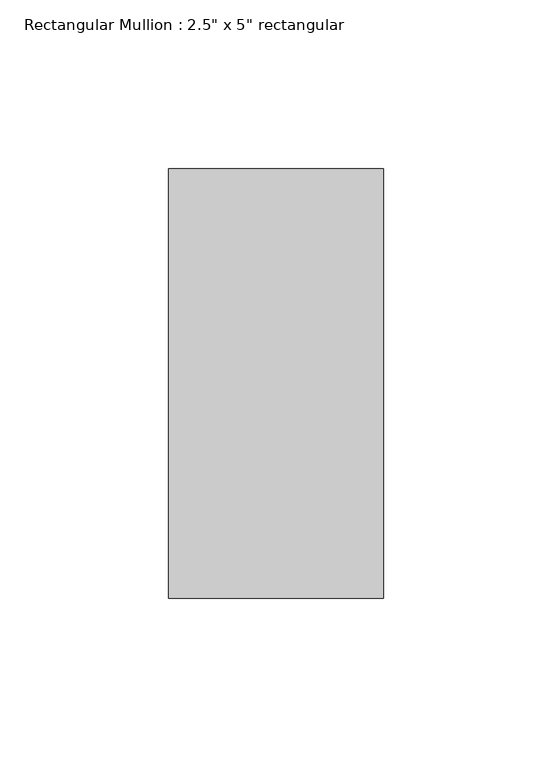
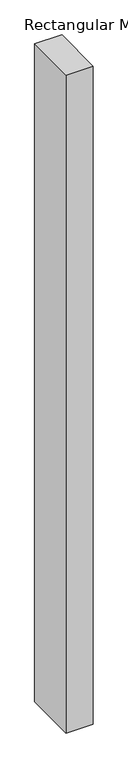
"""IFC4 building model written with IfcOpenShell, lengths in millimetres: member geometry."""

from ifc_helpers import new_model, si_unit, frame, origin, place, context, project, spatial, polyline, outline, extrude, source, transform, mapped, element, save


def member_1a0dfb12(model_context):
    return source(origin(), model_context, "Body", "SweptSolid", [
        extrude(outline(polyline([(31.75, 63.5), (31.75, -63.5), (-31.75, -63.5), (-31.75, 63.5), (31.75, 63.5)])), frame((0.0, 0.0, -1628.7655616), z_axis=(0.0, 0.0, 1.0), x_axis=(1.0, 0.0, 0.0)), (0.0, 0.0, 1.0), 1628.7655616),
    ])


if __name__ == "__main__":
    model = new_model("IFC4")
    model_context = context("Model", 3, world=origin())
    ifc_project = project(units=[si_unit("LENGTHUNIT", "METRE", prefix="MILLI")], contexts=[model_context])
    site = spatial("IfcSite", under=ifc_project)
    building = spatial("IfcBuilding", under=site)
    placement = place(None, origin())
    member_shape = member_1a0dfb12(model_context)
    element("IfcMember", 1, ObjectType="Rectangular Mullion : 2.5\" x 5\" rectangular", at=placement, inside=building, context=model_context, shape_type="MappedRepresentation", body=[
        mapped(member_shape, transform((0.0, 0.0, 0.0), x_axis=(1.0, 0.0, 0.0), y_axis=(0.0, 1.0, 0.0), z_axis=(0.0, 0.0, 1.0))),
    ])
    save(model, "model.ifc")

# Revit data of these elements
# Type "Rectangular Mullion : 2.5\" x 5\" rectangular"
#   built-in parameter 1007304 = 0.416667 (stored number, unit not read)
#   built-in parameter 1007301 = 0.104167 (stored number, unit not read)
#   built-in parameter 1007300 = 0.104167 (stored number, unit not read)
# Element 1 (IfcMember, "Rectangular Mullion : 2.5\" x 5\" rectangular")
#   Materials on its faces: "Aluminum"
# Materials
#   "Aluminum": class "Metal", colour RGB 247 247 247, transparency 0, Description = "Aluminum 6061", Cost = 0
